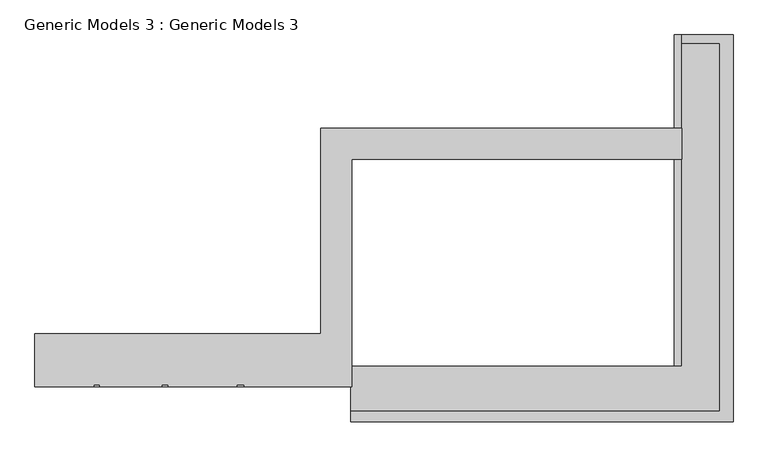
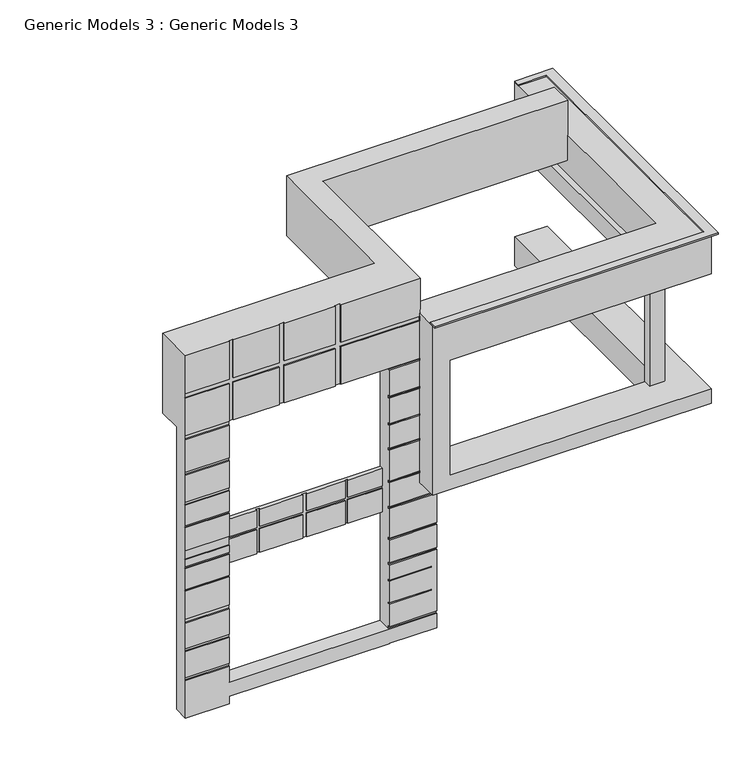
"""IFC4 building model written with IfcOpenShell, lengths in millimetres: proxy geometry, Generic Models 3 : Generic Models 3."""

from ifc_helpers import new_model, si_unit, frame, origin, place, context, project, spatial, polyline, outline, extrude, faceted_brep, source, transform, mapped, element, save


def generic_models_3_generic_models_3_8fccb6e9(model_context):
    return source(origin(), model_context, "Body", "SolidModel", [
        faceted_brep([(-13508.5518575, -15230.9378384, 3718.9773685), (-14205.0083823, -15230.9378384, 3718.9773685), (-14205.0083823, -15230.9378384, 3352.8), (-13508.5518575, -15230.9378384, 3352.8), (-13508.5518575, -15154.7378384, 3718.9773685), (-13508.5518575, -15154.7378384, 2802.4335272), (-16708.9518575, -15154.7378384, 2802.4335272), (-16708.9518575, -15154.7378384, 3718.9773685), (-16708.9518575, -15230.9378384, 3718.9773685), (-16030.1089145, -15230.9378384, 3718.9773685), (-16030.1089145, -15205.5378384, 3718.9773685), (-15961.8808572, -15205.5378384, 3718.9773685), (-15961.8808572, -15230.9378384, 3718.9773685), (-15108.7518575, -15230.9378384, 3718.9773685), (-15108.7518575, -15205.5378384, 3718.9773685), (-15023.7450696, -15205.5378384, 3718.9773685), (-15023.7450696, -15230.9378384, 3718.9773685), (-14250.4937538, -15230.9378384, 3718.9773685), (-14250.4937538, -15205.5378384, 3718.9773685), (-14205.0083823, -15205.5378384, 3718.9773685), (-16708.9518575, -15230.9378384, 2802.4335272), (-16708.9518575, -15230.9378384, 3300.7713885), (-16708.9518575, -15205.5378384, 3300.7713885), (-16708.9518575, -15205.5378384, 3352.8), (-16708.9518575, -15230.9378384, 3352.8), (-13508.5518575, -15230.9378384, 2802.4335272), (-14205.0083823, -15230.9378384, 2802.4335272), (-14205.0083823, -15205.5378384, 2802.4335272), (-14250.4937538, -15205.5378384, 2802.4335272), (-14250.4937538, -15230.9378384, 2802.4335272), (-15023.7450696, -15230.9378384, 2802.4335272), (-15023.7450696, -15205.5378384, 2802.4335272), (-15108.7518575, -15205.5378384, 2802.4335272), (-15108.7518575, -15230.9378384, 2802.4335272), (-15961.8808572, -15230.9378384, 2802.4335272), (-15961.8808572, -15205.5378384, 2802.4335272), (-16030.1089145, -15205.5378384, 2802.4335272), (-16030.1089145, -15230.9378384, 2802.4335272), (-13508.5518575, -15205.5378384, 3352.8), (-13508.5518575, -15205.5378384, 3300.7713885), (-13508.5518575, -15230.9378384, 3300.7713885), (-16030.1089145, -15205.5378384, 3352.8), (-16030.1089145, -15205.5378384, 3300.7713885), (-15961.8808572, -15205.5378384, 3300.7713885), (-15108.7518575, -15205.5378384, 3300.7713885), (-15023.7450696, -15205.5378384, 3300.7713885), (-14250.4937538, -15205.5378384, 3300.7713885), (-14205.0083823, -15205.5378384, 3300.7713885), (-14205.0083823, -15205.5378384, 3352.8), (-14250.4937538, -15205.5378384, 3352.8), (-15023.7450696, -15205.5378384, 3352.8), (-15108.7518575, -15205.5378384, 3352.8), (-15961.8808572, -15205.5378384, 3352.8), (-15961.8808572, -15230.9378384, 3352.8), (-16030.1089145, -15230.9378384, 3300.7713885), (-15023.7450696, -15230.9378384, 3352.8), (-15108.7518575, -15230.9378384, 3300.7713885), (-14250.4937538, -15230.9378384, 3300.7713885), (-14205.0083823, -15230.9378384, 3300.7713885), (-16030.1089145, -15230.9378384, 3352.8), (-14250.4937538, -15230.9378384, 3352.8), (-15023.7450696, -15230.9378384, 3300.7713885), (-15108.7518575, -15230.9378384, 3352.8), (-15961.8808572, -15230.9378384, 3300.7713885)], [[[0, 1, 2, 3]], [[4, 5, 6, 7]], [[4, 7, 8, 9, 10, 11, 12, 13, 14, 15, 16, 17, 18, 19, 1, 0]], [[7, 6, 20, 21, 22, 23, 24, 8]], [[6, 5, 25, 26, 27, 28, 29, 30, 31, 32, 33, 34, 35, 36, 37, 20]], [[5, 4, 0, 3, 38, 39, 40, 25]], [[11, 10, 41, 23, 22, 42, 36, 35, 43, 44, 32, 31, 45, 46, 28, 27, 47, 39, 38, 48, 19, 18, 49, 50, 15, 14, 51, 52]], [[12, 11, 52, 53]], [[37, 36, 42, 54]], [[16, 15, 50, 55]], [[33, 32, 44, 56]], [[1, 19, 48, 2]], [[29, 28, 46, 57]], [[39, 47, 58, 40]], [[23, 41, 59, 24]], [[26, 25, 40, 58]], [[17, 16, 55, 60]], [[30, 29, 57, 61]], [[13, 12, 53, 62]], [[34, 33, 56, 63]], [[9, 8, 24, 59]], [[20, 37, 54, 21]], [[35, 34, 63, 43]], [[10, 9, 59, 41]], [[31, 30, 61, 45]], [[14, 13, 62, 51]], [[27, 26, 58, 47]], [[18, 17, 60, 49]], [[46, 45, 61, 57]], [[44, 43, 63, 56]], [[42, 22, 21, 54]], [[52, 51, 62, 53]], [[50, 49, 60, 55]], [[48, 38, 3, 2]]]),
        extrude(outline(polyline([(-7423.6387627, -15826.0752214), (-7423.6387627, -10366.8378384), (-7984.0518575, -10366.8378384), (-7984.0518575, -10239.8378384), (-7224.7250276, -10239.8378384), (-7224.7250276, -15978.2714482), (-12898.9518575, -15978.2714482), (-12898.9518575, -15827.8378384), (-12707.2995814, -15827.8378384), (-12707.2995814, -15826.0752214), (-7423.6387627, -15826.0752214)])), frame((0.0, 0.0, 6931.8330206), z_axis=(0.0, 0.0, 1.0), x_axis=(1.0, 0.0, 0.0)), (0.0, 0.0, 1.0), 25.4),
        faceted_brep([(-12556.0518575, -15459.5378384, 6324.9002487), (-12886.2518575, -15459.5378384, 6324.9002487), (-12886.2518575, -15459.5378384, 6931.8330206), (-12898.9518575, -15459.5378384, 6931.8330206), (-12898.9518575, -15459.5378384, 7008.0330206), (-12886.2518575, -15459.5378384, 7008.0330206), (-12886.2518575, -15459.5378384, 7667.8975872), (-14480.3928241, -15459.5378384, 7667.8975872), (-14480.3928241, -15459.5378384, 6868.7554166), (-12898.9518575, -15459.5378384, 6868.7554166), (-12898.9518575, -15459.5378384, 6771.0215996), (-14480.3928241, -15459.5378384, 6771.0215996), (-14480.3928241, -15459.5378384, 5978.1644617), (-12898.9518575, -15459.5378384, 5978.1644617), (-12898.9518575, -15459.5378384, 5939.6307837), (-13508.5518575, -15459.5378384, 5939.6307837), (-13508.5518575, -15459.5378384, 5387.6635035), (-12898.9518575, -15459.5378384, 5387.6635035), (-12898.9518575, -15459.5378384, 5341.4833815), (-13508.5518575, -15459.5378384, 5341.4833815), (-13508.5518575, -15459.5378384, 4807.320436), (-12898.9518575, -15459.5378384, 4807.320436), (-12898.9518575, -15459.5378384, 4772.5931891), (-13508.5518575, -15459.5378384, 4772.5931891), (-13508.5518575, -15459.5378384, 4284.9730243), (-12898.9518575, -15459.5378384, 4284.9730243), (-12898.9518575, -15459.5378384, 4242.71261), (-13508.5518575, -15459.5378384, 4242.71261), (-13508.5518575, -15459.5378384, 3592.5523901), (-12898.9518575, -15459.5378384, 3592.5523901), (-12898.9518575, -15459.5378384, 3553.5427769), (-13508.5518575, -15459.5378384, 3553.5427769), (-13508.5518575, -15459.5378384, 3048.0), (-12556.0518575, -15459.5378384, 3048.0), (-16708.9518575, -15154.7378384, 0.0), (-17585.2518575, -15154.7378384, 0.0), (-17585.2518575, -15154.7378384, 5978.1644617), (-16708.9518575, -15154.7378384, 5978.1644617), (-16708.9518575, -15154.7378384, 458.502719), (-13508.5518575, -15154.7378384, 458.502719), (-13508.5518575, -15154.7378384, 5978.1644617), (-12886.2518575, -15154.7378384, 5978.1644617), (-12886.2518575, -15154.7378384, 6324.9002487), (-12556.0518575, -15154.7378384, 6324.9002487), (-12556.0518575, -15154.7378384, 154.9293516), (-13508.5518575, -15154.7378384, 154.9293516), (-13508.5518575, -15154.7378384, 153.702719), (-16708.9518575, -15154.7378384, 153.702719), (-17585.2518575, -15459.5378384, 0.0), (-17585.2518575, -15459.5378384, 794.199912), (-17585.2518575, -15434.1378384, 794.199912), (-17585.2518575, -15434.1378384, 858.4727196), (-17585.2518575, -15459.5378384, 858.4727196), (-17585.2518575, -15459.5378384, 1407.2636151), (-17585.2518575, -15434.1378384, 1407.2636151), (-17585.2518575, -15434.1378384, 1470.3856812), (-17585.2518575, -15459.5378384, 1470.3856812), (-17585.2518575, -15459.5378384, 2011.6752095), (-17585.2518575, -15434.1378384, 2011.6752095), (-17585.2518575, -15434.1378384, 2091.7649715), (-17585.2518575, -15459.5378384, 2091.7649715), (-17585.2518575, -15459.5378384, 2684.0752144), (-17585.2518575, -15434.1378384, 2684.0752144), (-17585.2518575, -15434.1378384, 2718.4882317), (-17585.2518575, -15459.5378384, 2718.4882317), (-17585.2518575, -15459.5378384, 3160.9413114), (-17585.2518575, -15434.1378384, 3160.9413114), (-17585.2518575, -15434.1378384, 3200.4), (-17585.2518575, -15459.5378384, 3200.4), (-17585.2518575, -15459.5378384, 3352.8), (-17585.2518575, -15434.1378384, 3352.8), (-17585.2518575, -15434.1378384, 3544.4006471), (-17585.2518575, -15459.5378384, 3544.4006471), (-17585.2518575, -15459.5378384, 4031.0990347), (-17585.2518575, -15434.1378384, 4031.0990347), (-17585.2518575, -15434.1378384, 4077.6512698), (-17585.2518575, -15459.5378384, 4077.6512698), (-17585.2518575, -15459.5378384, 4503.9707636), (-17585.2518575, -15434.1378384, 4503.9707636), (-17585.2518575, -15434.1378384, 4572.0), (-17585.2518575, -15459.5378384, 4572.0), (-17585.2518575, -15459.5378384, 5144.3785801), (-17585.2518575, -15434.1378384, 5144.3785801), (-17585.2518575, -15434.1378384, 5201.9683032), (-17585.2518575, -15459.5378384, 5201.9683032), (-17585.2518575, -15459.5378384, 5895.6635035), (-17585.2518575, -15434.1378384, 5895.6635035), (-17585.2518575, -15434.1378384, 5978.1644617), (-17585.2518575, -15459.5378384, 5978.1644617), (-17585.2518575, -15459.5378384, 6771.0215996), (-17585.2518575, -15434.1378384, 6771.0215996), (-17585.2518575, -15434.1378384, 6868.7554166), (-17585.2518575, -15459.5378384, 6868.7554166), (-17585.2518575, -15459.5378384, 7667.8975872), (-17585.2518575, -14672.1378384, 7667.8975872), (-17585.2518575, -14672.1378384, 5978.1644617), (-16708.9518575, -15459.5378384, 0.0), (-16708.9518575, -15459.5378384, 6771.0215996), (-16708.9518575, -15459.5378384, 5978.1644617), (-16708.9518575, -15434.1378384, 5978.1644617), (-16708.9518575, -15434.1378384, 6771.0215996), (-13508.5518575, -15434.1378384, 458.502719), (-13508.5518575, -15434.1378384, 509.302719), (-13508.5518575, -15459.5378384, 509.302719), (-13508.5518575, -15459.5378384, 985.4099086), (-13508.5518575, -15434.1378384, 985.4099086), (-13508.5518575, -15434.1378384, 1011.4163174), (-13508.5518575, -15459.5378384, 1011.4163174), (-13508.5518575, -15459.5378384, 1470.3856812), (-13508.5518575, -15434.1378384, 1470.3856812), (-13508.5518575, -15434.1378384, 1495.7856812), (-13508.5518575, -15459.5378384, 1495.7856812), (-13508.5518575, -15459.5378384, 1814.3641889), (-13508.5518575, -15434.1378384, 1814.3641889), (-13508.5518575, -15434.1378384, 1859.8754043), (-13508.5518575, -15459.5378384, 1859.8754043), (-13508.5518575, -15459.5378384, 2340.993967), (-13508.5518575, -15434.1378384, 2340.993967), (-13508.5518575, -15434.1378384, 2386.5051824), (-13508.5518575, -15459.5378384, 2386.5051824), (-13508.5518575, -15459.5378384, 3004.1573912), (-13508.5518575, -15434.1378384, 3004.1573912), (-13508.5518575, -15434.1378384, 3048.0), (-13508.5518575, -15434.1378384, 3553.5427769), (-13508.5518575, -15434.1378384, 3592.5523901), (-13508.5518575, -15434.1378384, 4242.71261), (-13508.5518575, -15434.1378384, 4284.9730243), (-13508.5518575, -15434.1378384, 4772.5931891), (-13508.5518575, -15434.1378384, 4807.320436), (-13508.5518575, -15434.1378384, 5341.4833815), (-13508.5518575, -15434.1378384, 5387.6635035), (-13508.5518575, -15434.1378384, 5939.6307837), (-13508.5518575, -15434.1378384, 5978.1644617), (-12556.0518575, -15459.5378384, 154.9293516), (-13508.5518575, -15459.5378384, 154.9293516), (-12556.0518575, -15434.1378384, 3048.0), (-12556.0518575, -15434.1378384, 3004.1573912), (-12556.0518575, -15459.5378384, 3004.1573912), (-12556.0518575, -15459.5378384, 2386.5051824), (-12556.0518575, -15434.1378384, 2386.5051824), (-12556.0518575, -15434.1378384, 2340.993967), (-12556.0518575, -15459.5378384, 2340.993967), (-12556.0518575, -15459.5378384, 1859.8754043), (-12556.0518575, -15434.1378384, 1859.8754043), (-12556.0518575, -15434.1378384, 1814.3641889), (-12556.0518575, -15459.5378384, 1814.3641889), (-12556.0518575, -15459.5378384, 509.302719), (-12556.0518575, -15434.1378384, 509.302719), (-12556.0518575, -15434.1378384, 458.502719), (-12556.0518575, -15459.5378384, 458.502719), (-16708.9518575, -15459.5378384, 7667.8975872), (-16708.9518575, -15434.1378384, 7667.8975872), (-16625.0280912, -15434.1378384, 7667.8975872), (-16625.0280912, -15459.5378384, 7667.8975872), (-15703.0964673, -15459.5378384, 7667.8975872), (-15703.0964673, -15434.1378384, 7667.8975872), (-15605.0186349, -15434.1378384, 7667.8975872), (-15605.0186349, -15459.5378384, 7667.8975872), (-14591.5477008, -15459.5378384, 7667.8975872), (-14591.5477008, -15434.1378384, 7667.8975872), (-14480.3928241, -15434.1378384, 7667.8975872), (-12886.2518575, -12081.3378384, 7667.8975872), (-7984.0518575, -12081.3378384, 7667.8975872), (-7984.0518575, -11624.1378384, 7667.8975872), (-13343.4518575, -11624.1378384, 7667.8975872), (-13343.4518575, -14672.1378384, 7667.8975872), (-12886.2518575, -14672.1378384, 5978.1644617), (-12898.9518575, -15434.1378384, 5978.1644617), (-14480.3928241, -15434.1378384, 5978.1644617), (-14591.5477008, -15434.1378384, 5978.1644617), (-14591.5477008, -15459.5378384, 5978.1644617), (-15605.0186349, -15459.5378384, 5978.1644617), (-15605.0186349, -15434.1378384, 5978.1644617), (-15703.0964673, -15434.1378384, 5978.1644617), (-15703.0964673, -15459.5378384, 5978.1644617), (-16625.0280912, -15459.5378384, 5978.1644617), (-16625.0280912, -15434.1378384, 5978.1644617), (-12886.2518575, -14672.1378384, 6400.8), (-12886.2518575, -12081.3378384, 6400.8), (-12886.2518575, -15154.7378384, 7008.0330206), (-12886.2518575, -15154.7378384, 6931.8330206), (-13343.4518575, -14672.1378384, 6400.8), (-16708.9518575, -15459.5378384, 458.502719), (-13508.5518575, -15459.5378384, 153.702719), (-16708.9518575, -15459.5378384, 153.702719), (-13343.4518575, -11624.1378384, 6400.8), (-7984.0518575, -11624.1378384, 6400.8), (-7984.0518575, -12081.3378384, 6400.8), (-16625.0280912, -15459.5378384, 6868.7554166), (-16625.0280912, -15434.1378384, 6868.7554166), (-15703.0964673, -15459.5378384, 6771.0215996), (-15703.0964673, -15434.1378384, 6771.0215996), (-15605.0186349, -15459.5378384, 6868.7554166), (-15605.0186349, -15434.1378384, 6868.7554166), (-14591.5477008, -15459.5378384, 6771.0215996), (-14591.5477008, -15434.1378384, 6771.0215996), (-14480.3928241, -15434.1378384, 6868.7554166), (-16708.9518575, -15459.5378384, 5895.6635035), (-16708.9518575, -15434.1378384, 5895.6635035), (-12898.9518575, -15434.1378384, 6868.7554166), (-12898.9518575, -15434.1378384, 6771.0215996), (-14480.3928241, -15434.1378384, 6771.0215996), (-16708.9518575, -15459.5378384, 6868.7554166), (-16708.9518575, -15434.1378384, 6868.7554166), (-16708.9518575, -15459.5378384, 5144.3785801), (-16708.9518575, -15434.1378384, 5144.3785801), (-16708.9518575, -15459.5378384, 5201.9683032), (-16708.9518575, -15434.1378384, 5201.9683032), (-16708.9518575, -15459.5378384, 4503.9707636), (-16708.9518575, -15434.1378384, 4503.9707636), (-16708.9518575, -15459.5378384, 4572.0), (-16708.9518575, -15434.1378384, 4572.0), (-16708.9518575, -15459.5378384, 4031.0990347), (-16708.9518575, -15434.1378384, 4031.0990347), (-16708.9518575, -15459.5378384, 4077.6512698), (-16708.9518575, -15434.1378384, 4077.6512698), (-16708.9518575, -15459.5378384, 3352.8), (-16708.9518575, -15434.1378384, 3352.8), (-16708.9518575, -15459.5378384, 3544.4006471), (-16708.9518575, -15434.1378384, 3544.4006471), (-16708.9518575, -15459.5378384, 3160.9413114), (-16708.9518575, -15434.1378384, 3160.9413114), (-16708.9518575, -15459.5378384, 3200.4), (-16708.9518575, -15434.1378384, 3200.4), (-16708.9518575, -15459.5378384, 2684.0752144), (-16708.9518575, -15434.1378384, 2684.0752144), (-16708.9518575, -15459.5378384, 2718.4882317), (-16708.9518575, -15434.1378384, 2718.4882317), (-12898.9518575, -15434.1378384, 5939.6307837), (-12898.9518575, -15434.1378384, 5387.6635035), (-12898.9518575, -15434.1378384, 5341.4833815), (-12898.9518575, -15434.1378384, 4807.320436), (-12898.9518575, -15434.1378384, 4772.5931891), (-12898.9518575, -15434.1378384, 4284.9730243), (-12898.9518575, -15434.1378384, 4242.71261), (-12898.9518575, -15434.1378384, 3592.5523901), (-12898.9518575, -15434.1378384, 3553.5427769), (-12670.3518575, -15459.5378384, 1470.3856812), (-12670.3518575, -15459.5378384, 1495.7856812), (-12670.3518575, -15434.1378384, 1495.7856812), (-12670.3518575, -15434.1378384, 1470.3856812), (-12670.3518575, -15459.5378384, 985.4099086), (-12670.3518575, -15459.5378384, 1011.4163174), (-12670.3518575, -15434.1378384, 1011.4163174), (-12670.3518575, -15434.1378384, 985.4099086), (-16708.9518575, -15459.5378384, 2011.6752095), (-16708.9518575, -15434.1378384, 2011.6752095), (-16708.9518575, -15459.5378384, 2091.7649715), (-16708.9518575, -15434.1378384, 2091.7649715), (-16708.9518575, -15459.5378384, 1407.2636151), (-16708.9518575, -15434.1378384, 1407.2636151), (-16708.9518575, -15459.5378384, 1470.3856812), (-16708.9518575, -15434.1378384, 1470.3856812), (-16708.9518575, -15459.5378384, 794.199912), (-16708.9518575, -15434.1378384, 794.199912), (-16708.9518575, -15459.5378384, 858.4727196), (-16708.9518575, -15434.1378384, 858.4727196), (-14591.5477008, -15459.5378384, 6868.7554166), (-15605.0186349, -15459.5378384, 6771.0215996), (-15703.0964673, -15459.5378384, 6868.7554166), (-16625.0280912, -15459.5378384, 6771.0215996), (-16625.0280912, -15434.1378384, 6771.0215996), (-15605.0186349, -15434.1378384, 6771.0215996), (-14591.5477008, -15434.1378384, 6868.7554166), (-15703.0964673, -15434.1378384, 6868.7554166), (-12898.9518575, -15154.7378384, 7008.0330206), (-12898.9518575, -15154.7378384, 6931.8330206)], [[[0, 1, 2, 3, 4, 5, 6, 7, 8, 9, 10, 11, 12, 13, 14, 15, 16, 17, 18, 19, 20, 21, 22, 23, 24, 25, 26, 27, 28, 29, 30, 31, 32, 33]], [[34, 35, 36, 37, 38, 39, 40, 41, 42, 43, 44, 45, 46, 47]], [[36, 35, 48, 49, 50, 51, 52, 53, 54, 55, 56, 57, 58, 59, 60, 61, 62, 63, 64, 65, 66, 67, 68, 69, 70, 71, 72, 73, 74, 75, 76, 77, 78, 79, 80, 81, 82, 83, 84, 85, 86, 87, 88, 89, 90, 91, 92, 93, 94, 95]], [[96, 48, 35, 34]], [[97, 98, 99, 100]], [[1, 0, 43, 42]], [[40, 39, 101, 102, 103, 104, 105, 106, 107, 108, 109, 110, 111, 112, 113, 114, 115, 116, 117, 118, 119, 120, 121, 122, 32, 31, 123, 124, 28, 27, 125, 126, 24, 23, 127, 128, 20, 19, 129, 130, 16, 15, 131, 132]], [[133, 134, 45, 44]], [[44, 43, 0, 33, 135, 136, 137, 138, 139, 140, 141, 142, 143, 144, 145, 146, 147, 148, 149, 133]], [[94, 93, 150, 151, 152, 153, 154, 155, 156, 157, 158, 159, 160, 7, 6, 161, 162, 163, 164, 165]], [[37, 36, 95, 166, 41, 40, 132, 167, 13, 12, 168, 169, 170, 171, 172, 173, 174, 175, 176, 99]], [[42, 41, 166, 177, 178, 161, 6, 5, 179, 180, 2, 1]], [[95, 94, 165, 181, 177, 166]], [[39, 38, 182, 149, 148, 101]], [[183, 184, 47, 46]], [[134, 183, 46, 45]], [[178, 177, 181, 185, 186, 187]], [[165, 164, 185, 181]], [[163, 162, 187, 186]], [[164, 163, 186, 185]], [[162, 161, 178, 187]], [[102, 101, 148, 147]], [[188, 153, 152, 189]], [[190, 174, 173, 191]], [[192, 157, 156, 193]], [[194, 170, 169, 195]], [[8, 7, 160, 196]], [[98, 88, 87, 99]], [[85, 197, 198, 86]], [[10, 9, 199, 200]], [[11, 10, 200, 201]], [[202, 92, 91, 203]], [[81, 204, 205, 82]], [[206, 84, 83, 207]], [[77, 208, 209, 78]], [[210, 80, 79, 211]], [[73, 212, 213, 74]], [[214, 76, 75, 215]], [[69, 216, 217, 70]], [[218, 72, 71, 219]], [[65, 220, 221, 66]], [[222, 68, 67, 223]], [[61, 224, 225, 62]], [[226, 64, 63, 227]], [[14, 13, 167, 228]], [[15, 14, 228, 131]], [[18, 17, 229, 230]], [[19, 18, 230, 129]], [[17, 16, 130, 229]], [[22, 21, 231, 232]], [[23, 22, 232, 127]], [[21, 20, 128, 231]], [[26, 25, 233, 234]], [[27, 26, 234, 125]], [[25, 24, 126, 233]], [[30, 29, 235, 236]], [[31, 30, 236, 123]], [[29, 28, 124, 235]], [[120, 137, 136, 121]], [[33, 32, 122, 135]], [[116, 141, 140, 117]], [[138, 119, 118, 139]], [[112, 145, 144, 113]], [[142, 115, 114, 143]], [[237, 238, 239, 240]], [[108, 237, 240, 109]], [[238, 111, 110, 239]], [[241, 242, 243, 244]], [[104, 241, 244, 105]], [[242, 107, 106, 243]], [[57, 245, 246, 58]], [[247, 60, 59, 248]], [[53, 249, 250, 54]], [[251, 56, 55, 252]], [[49, 253, 254, 50]], [[255, 52, 51, 256]], [[146, 103, 102, 147]], [[138, 137, 120, 119]], [[142, 141, 116, 115]], [[146, 145, 112, 111, 238, 237, 108, 107, 242, 241, 104, 103]], [[158, 157, 192, 257]], [[171, 170, 194, 258]], [[154, 153, 188, 259]], [[175, 174, 190, 260]], [[150, 93, 92, 202]], [[98, 97, 89, 88]], [[206, 197, 85, 84]], [[210, 204, 81, 80]], [[214, 208, 77, 76]], [[218, 212, 73, 72]], [[222, 216, 69, 68]], [[226, 220, 65, 64]], [[247, 224, 61, 60]], [[251, 245, 57, 56]], [[255, 249, 53, 52]], [[48, 96, 184, 183, 134, 133, 149, 182, 253, 49]], [[150, 202, 203, 151]], [[184, 96, 34, 47]], [[38, 37, 99, 198, 197, 206, 207, 205, 204, 210, 211, 209, 208, 214, 215, 213, 212, 218, 219, 217, 216, 222, 223, 221, 220, 226, 227, 225, 224, 247, 248, 246, 245, 251, 252, 250, 249, 255, 256, 254, 253, 182]], [[114, 113, 144, 143]], [[118, 117, 140, 139]], [[122, 121, 136, 135]], [[110, 109, 240, 239]], [[106, 105, 244, 243]], [[124, 123, 236, 235]], [[126, 125, 234, 233]], [[128, 127, 232, 231]], [[130, 129, 230, 229]], [[132, 131, 228, 167]], [[51, 50, 254, 256]], [[55, 54, 250, 252]], [[59, 58, 246, 248]], [[63, 62, 225, 227]], [[67, 66, 221, 223]], [[71, 70, 217, 219]], [[75, 74, 213, 215]], [[79, 78, 209, 211]], [[83, 82, 205, 207]], [[91, 90, 100, 99, 176, 261, 191, 173, 172, 262, 195, 169, 168, 201, 200, 199, 196, 160, 159, 263, 193, 156, 155, 264, 189, 152, 151, 203]], [[87, 86, 198, 99]], [[175, 260, 261, 176]], [[154, 259, 264, 155]], [[171, 258, 262, 172]], [[158, 257, 263, 159]], [[12, 11, 201, 168]], [[258, 194, 195, 262]], [[260, 190, 191, 261]], [[89, 97, 100, 90]], [[259, 188, 189, 264]], [[257, 192, 193, 263]], [[9, 8, 196, 199]], [[265, 179, 5, 4]], [[266, 3, 2, 180]], [[266, 265, 4, 3]], [[265, 266, 180, 179]]]),
        faceted_brep([(-7326.3250276, -15916.2524677, 6096.0), (-7326.3250276, -15916.2524677, 6931.8330206), (-12898.9518575, -15916.2524677, 6931.8330206), (-12898.9518575, -15916.2524677, 3352.8), (-7326.3250276, -15916.2524677, 3352.8), (-7326.3250276, -15916.2524677, 3657.6), (-12556.0518575, -15916.2524677, 3657.6), (-12556.0518575, -15916.2524677, 6096.0), (-12898.9518575, -15154.7378384, 6931.8330206), (-12707.2995814, -15154.7378384, 6931.8330206), (-7984.0518575, -15154.7378384, 6931.8330206), (-7984.0518575, -15154.7378384, 6096.0), (-8098.3518575, -15154.7378384, 6096.0), (-8098.3518575, -15154.7378384, 5714.786093), (-7907.8518575, -15154.7378384, 5714.786093), (-7907.8518575, -15154.7378384, 3657.6), (-7984.0518575, -15154.7378384, 3657.6), (-7984.0518575, -15154.7378384, 3048.0), (-12556.0518575, -15154.7378384, 3048.0), (-12556.0518575, -15154.7378384, 3352.8), (-12898.9518575, -15154.7378384, 3352.8), (-8212.6518575, -15154.7378384, 5714.786093), (-12302.0518575, -15154.7378384, 5714.786093), (-12302.0518575, -15154.7378384, 3657.6), (-8212.6518575, -15154.7378384, 3657.6), (-12898.9518575, -15827.8378384, 6931.8330206), (-7326.3250276, -10239.8378384, 6931.8330206), (-7984.0518575, -10239.8378384, 6931.8330206), (-7326.3250276, -10239.8378384, 6096.0), (-12556.0518575, -15317.4823236, 6096.0), (-7907.8518575, -15317.4823236, 6096.0), (-7907.8518575, -10239.8378384, 6096.0), (-7984.0518575, -10239.8378384, 6096.0), (-7907.8518575, -10239.8378384, 5714.786093), (-8098.3518575, -10239.8378384, 5714.786093), (-8098.3518575, -10239.8378384, 6096.0), (-12556.0518575, -15459.5378384, 3352.8), (-12556.0518575, -15459.5378384, 3048.0), (-7679.2518575, -15459.5378384, 3048.0), (-7679.2518575, -15459.5378384, 3352.8), (-12556.0518575, -15434.1378384, 3048.0), (-7984.0518575, -10239.8378384, 3048.0), (-7679.2518575, -10239.8378384, 3048.0), (-7679.2518575, -10239.8378384, 3352.8), (-7984.0518575, -10239.8378384, 3657.6), (-7326.3250276, -10239.8378384, 3657.6), (-7326.3250276, -10239.8378384, 3352.8), (-7907.8518575, -15317.4823236, 3657.6), (-8212.6518575, -15317.4823236, 3657.6), (-12302.0518575, -15317.4823236, 3657.6), (-12556.0518575, -15317.4823236, 3657.6), (-12302.0518575, -15317.4823236, 5714.786093), (-8212.6518575, -15317.4823236, 5714.786093)], [[[0, 1, 2, 3, 4, 5, 6, 7]], [[8, 9, 10, 11, 12, 13, 14, 15, 16, 17, 18, 19, 20], [21, 22, 23, 24]], [[10, 9, 8, 25, 2, 1, 26, 27]], [[2, 25, 8, 20, 3]], [[28, 0, 7, 29, 30, 31]], [[26, 1, 0, 28]], [[27, 32, 11, 10]], [[26, 28, 31, 33, 34, 35, 32, 27]], [[36, 37, 38, 39]], [[37, 36, 19, 18, 40]], [[18, 17, 41, 42, 38, 37, 40]], [[39, 38, 42, 43]], [[41, 17, 16, 44]], [[43, 42, 41, 44, 45, 46]], [[5, 45, 44, 16, 15, 47, 48, 24, 23, 49, 50, 6]], [[3, 20, 19, 36, 39, 43, 46, 4]], [[45, 5, 4, 46]], [[7, 6, 50, 29]], [[51, 52, 48, 47, 30, 29, 50, 49]], [[52, 51, 22, 21]], [[30, 47, 15, 14, 33, 31]], [[21, 24, 48, 52]], [[23, 22, 51, 49]], [[35, 12, 11, 32]], [[34, 33, 14, 13]], [[35, 34, 13, 12]]]),
    ])


if __name__ == "__main__":
    model = new_model("IFC4")
    model_context = context("Model", 3, world=origin())
    ifc_project = project(units=[si_unit("LENGTHUNIT", "METRE", prefix="MILLI")], contexts=[model_context])
    site = spatial("IfcSite", under=ifc_project)
    building = spatial("IfcBuilding", under=site)
    placement = place(None, origin())
    generic_models_3_generic_models_3_shape = generic_models_3_generic_models_3_8fccb6e9(model_context)
    element("IfcBuildingElementProxy", 1, Name="Generic Models 3 : Generic Models 3", ObjectType="Generic Models 3 : Generic Models 3", at=placement, inside=building, context=model_context, shape_type="MappedRepresentation", body=[
        mapped(generic_models_3_generic_models_3_shape, transform((0.0, 0.0, 0.0), x_axis=(1.0, 0.0, 0.0), y_axis=(0.0, 1.0, 0.0), z_axis=(0.0, 0.0, 1.0))),
    ])
    save(model, "model.ifc")
